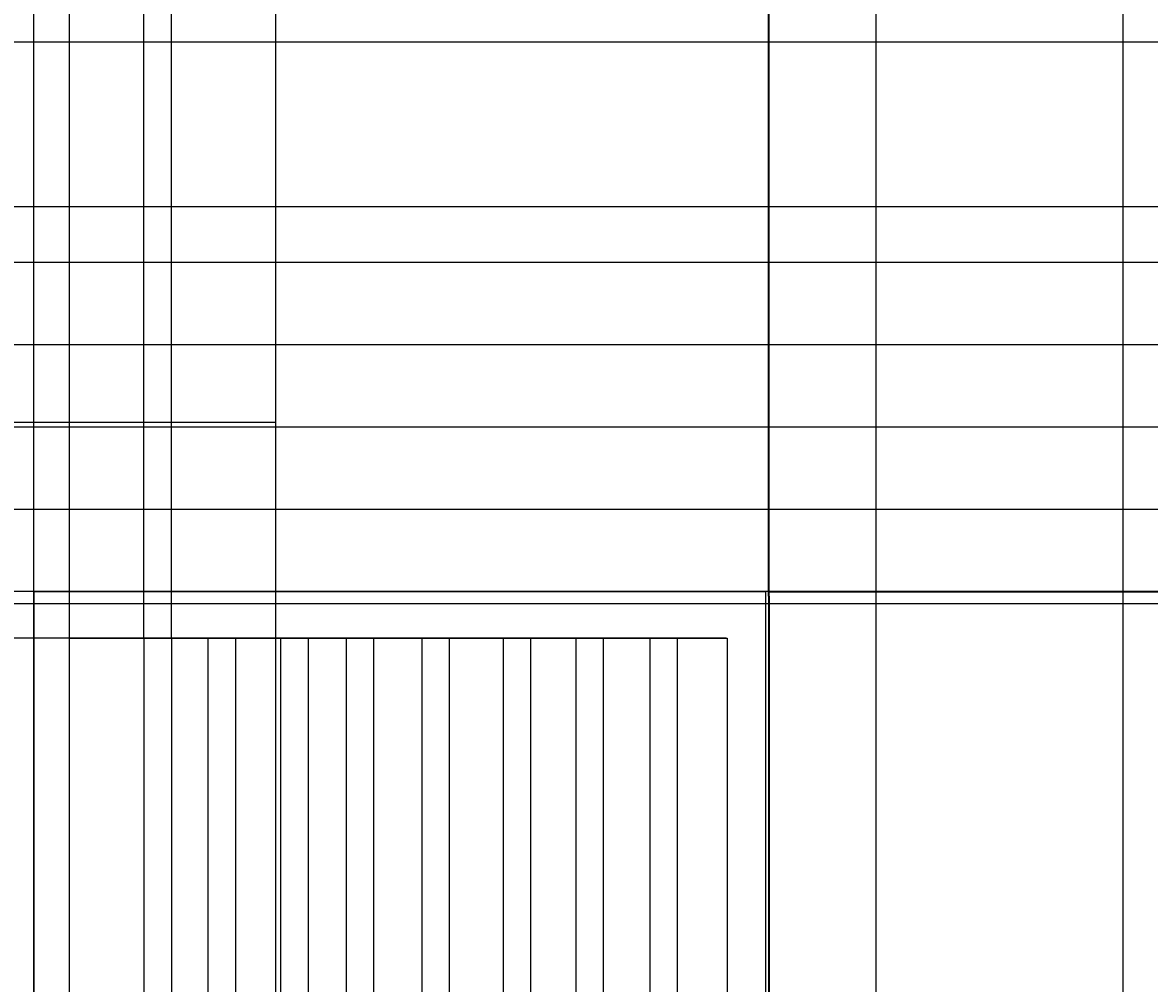
# Model space of a CAD drawing. Units: inches. Extents: x -13 to 809, y 112 to 656.
# Tile 12 of 55: x 257 to 339, y 182 to 252. Entities that reach past the tile are written whole.
import ezdxf

# ---------------------------------------------------------------- set-up
doc = ezdxf.new("R2010")
doc.units = ezdxf.units.IN
doc.header["$MEASUREMENT"] = 0
for name, color, linetype, lineweight in [('A-ANNO-DIMS', 2, 'Continuous', 18), ('A-DOOR', 4, 'Continuous', 25), ('A-ELEV', 7, 'Continuous', 35), ('A-GLAZ', 4, 'Continuous', 25)]:
    doc.layers.add(name, color=color, linetype=linetype, lineweight=lineweight)
doc.styles.get("Standard").update_dxf_attribs({"font": 'arial.ttf'})
doc.dimstyles.get("Standard").update_dxf_attribs({"dimtxt": 0.625, "dimasz": 0.18, "dimexe": 0.18, "dimexo": 0.0625, "dimgap": 0.09, "dimtad": 0, "dimtih": 1, "dimtoh": 1, "dimdec": 4, "dimzin": 0, "dimdsep": 46, "dimlunit": 4, "dimtxsty": 'Standard', "dimcen": 0.09, "dimadec": 0, "dimazin": 0, "dimtfac": 1, "dimtdec": 4, "dimtofl": 0, "dimtmove": 0, "dimatfit": 3, "dimfxl": 1, "dimtolj": 1, "dimtzin": 0, "dimarcsym": 0})

# ---------------------------------------------------------------- blocks, each defined once
blk = doc.blocks.new('*D15')
at = {"layer": 'A-ANNO-DIMS', "color": 0, "lineweight": -2, "transparency": 16777216}
for p, q in [((210.079, 223.038), (210.079, 112.34)), ((258.102, 210.722), (258.102, 112.34)), ((210.259, 112.52), (232.937, 112.52)), ((257.922, 112.52), (235.245, 112.52))]:
    blk.add_line(p, q, dxfattribs=at)
at = {"layer": 'A-ANNO-DIMS', "color": 0, "transparency": 16777216}
for points in [[(210.259, 112.55), (210.259, 112.49), (210.079, 112.52)], [(257.922, 112.55), (257.922, 112.49), (258.102, 112.52)]]:
    blk.add_solid(points, dxfattribs=at)
at = {"layer": 'Defpoints', "color": 0, "transparency": 16777216}
for p in [(210.079, 223.1), (258.102, 210.785), (258.102, 112.52)]:
    blk.add_point(p, dxfattribs=at)
at = {"layer": 'A-ANNO-DIMS', "color": 0, "transparency": 16777216, "insert": (234.091, 112.52), "char_height": 0.625, "attachment_point": 5}
blk.add_mtext('\\A1;48.02', dxfattribs=at)
blk = doc.blocks.new('*D16')
at = {"layer": 'A-ANNO-DIMS', "color": 0, "lineweight": -2, "transparency": 16777216}
for p, q in [((275.715, 223.038), (275.715, 112.34)), ((258.102, 210.722), (258.102, 112.34)), ((258.282, 112.52), (265.554, 112.52)), ((275.535, 112.52), (268.263, 112.52))]:
    blk.add_line(p, q, dxfattribs=at)
at = {"layer": 'A-ANNO-DIMS', "color": 0, "transparency": 16777216}
for points in [[(258.282, 112.55), (258.282, 112.49), (258.102, 112.52)], [(275.535, 112.55), (275.535, 112.49), (275.715, 112.52)]]:
    blk.add_solid(points, dxfattribs=at)
at = {"layer": 'Defpoints', "color": 0, "transparency": 16777216}
for p in [(275.715, 223.1), (258.102, 210.785), (275.715, 112.52)]:
    blk.add_point(p, dxfattribs=at)
at = {"layer": 'A-ANNO-DIMS', "color": 0, "transparency": 16777216, "insert": (266.908, 112.52), "char_height": 0.625, "attachment_point": 5}
blk.add_mtext('\\A1;17.612', dxfattribs=at)
blk = doc.blocks.new('*D17')
at = {"layer": 'A-ANNO-DIMS', "color": 0, "lineweight": -2, "transparency": 16777216}
for p, q in [((275.715, 223.038), (275.715, 112.34)), ((311.463, 210.722), (311.463, 112.34)), ((275.895, 112.52), (292.442, 112.52)), ((311.283, 112.52), (294.735, 112.52))]:
    blk.add_line(p, q, dxfattribs=at)
at = {"layer": 'A-ANNO-DIMS', "color": 0, "transparency": 16777216}
for points in [[(275.895, 112.55), (275.895, 112.49), (275.715, 112.52)], [(311.283, 112.55), (311.283, 112.49), (311.463, 112.52)]]:
    blk.add_solid(points, dxfattribs=at)
at = {"layer": 'Defpoints', "color": 0, "transparency": 16777216}
for p in [(275.715, 223.1), (311.463, 210.785), (311.463, 112.52)]:
    blk.add_point(p, dxfattribs=at)
at = {"layer": 'A-ANNO-DIMS', "color": 0, "transparency": 16777216, "insert": (293.589, 112.52), "char_height": 0.625, "attachment_point": 5}
blk.add_mtext('\\A1;35.75', dxfattribs=at)
blk = doc.blocks.new('*D18')
at = {"layer": 'A-ANNO-DIMS', "color": 0, "lineweight": -2, "transparency": 16777216}
for p, q in [((337.507, 306.457), (337.507, 112.34)), ((311.463, 210.722), (311.463, 112.34)), ((311.643, 112.52), (323.09, 112.52)), ((337.327, 112.52), (325.88, 112.52))]:
    blk.add_line(p, q, dxfattribs=at)
at = {"layer": 'A-ANNO-DIMS', "color": 0, "transparency": 16777216}
for points in [[(311.643, 112.55), (311.643, 112.49), (311.463, 112.52)], [(337.327, 112.55), (337.327, 112.49), (337.507, 112.52)]]:
    blk.add_solid(points, dxfattribs=at)
at = {"layer": 'Defpoints', "color": 0, "transparency": 16777216}
for p in [(337.507, 306.52), (311.463, 210.785), (337.507, 112.52)]:
    blk.add_point(p, dxfattribs=at)
at = {"layer": 'A-ANNO-DIMS', "color": 0, "transparency": 16777216, "insert": (324.485, 112.52), "char_height": 0.625, "attachment_point": 5}
blk.add_mtext('\\A1;26.045', dxfattribs=at)
blk = doc.blocks.new('*D19')
at = {"layer": 'A-ANNO-DIMS', "color": 0, "lineweight": -2, "transparency": 16777216}
for p, q in [((337.507, 306.457), (337.507, 112.34)), ((365.938, 210.722), (365.938, 112.34)), ((337.687, 112.52), (350.573, 112.52)), ((365.758, 112.52), (352.873, 112.52))]:
    blk.add_line(p, q, dxfattribs=at)
at = {"layer": 'A-ANNO-DIMS', "color": 0, "transparency": 16777216}
for points in [[(337.687, 112.55), (337.687, 112.49), (337.507, 112.52)], [(365.758, 112.55), (365.758, 112.49), (365.938, 112.52)]]:
    blk.add_solid(points, dxfattribs=at)
at = {"layer": 'Defpoints', "color": 0, "transparency": 16777216}
for p in [(337.507, 306.52), (365.938, 210.785), (365.938, 112.52)]:
    blk.add_point(p, dxfattribs=at)
at = {"layer": 'A-ANNO-DIMS', "color": 0, "transparency": 16777216, "insert": (351.723, 112.52), "char_height": 0.625, "attachment_point": 5}
blk.add_mtext('\\A1;28.43', dxfattribs=at)
blk = doc.blocks.new('*D45')
at = {"layer": 'A-ANNO-DIMS', "color": 0, "lineweight": -2, "transparency": 16777216}
for p, q in [((275.652, 270.602), (-12.099, 270.602)), ((-11.919, 270.422), (-11.919, 247.259)), ((-11.919, 223.28), (-11.919, 246.443)), ((275.652, 223.1), (-12.099, 223.1))]:
    blk.add_line(p, q, dxfattribs=at)
at = {"layer": 'A-ANNO-DIMS', "color": 0, "transparency": 16777216}
for points in [[(-11.949, 270.422), (-11.889, 270.422), (-11.919, 270.602)], [(-11.949, 223.28), (-11.889, 223.28), (-11.919, 223.1)]]:
    blk.add_solid(points, dxfattribs=at)
at = {"layer": 'Defpoints', "color": 0, "transparency": 16777216}
for p in [(-11.919, 270.602), (275.715, 270.602), (275.715, 223.1)]:
    blk.add_point(p, dxfattribs=at)
at = {"layer": 'A-ANNO-DIMS', "color": 0, "transparency": 16777216, "insert": (-11.919, 246.851), "char_height": 0.625, "attachment_point": 5}
blk.add_mtext('\\A1;47.5', dxfattribs=at)
blk = doc.blocks.new('*D49')
at = {"layer": 'A-ANNO-DIMS', "color": 0, "lineweight": -2, "transparency": 16777216}
for p, q in [((590.946, 250.843), (-12.099, 250.843)), ((-11.919, 250.663), (-11.919, 245.247)), ((-11.919, 239.023), (-11.919, 244.439)), ((590.946, 238.843), (-12.099, 238.843))]:
    blk.add_line(p, q, dxfattribs=at)
at = {"layer": 'A-ANNO-DIMS', "color": 0, "transparency": 16777216}
for points in [[(-11.949, 250.663), (-11.889, 250.663), (-11.919, 250.843)], [(-11.949, 239.023), (-11.889, 239.023), (-11.919, 238.843)]]:
    blk.add_solid(points, dxfattribs=at)
at = {"layer": 'Defpoints', "color": 0, "transparency": 16777216}
for p in [(-11.919, 250.843), (591.008, 250.843), (591.008, 238.843)]:
    blk.add_point(p, dxfattribs=at)
at = {"layer": 'A-ANNO-DIMS', "color": 0, "transparency": 16777216, "insert": (-11.919, 244.843), "char_height": 0.625, "attachment_point": 5}
blk.add_mtext('\\A1;12', dxfattribs=at)
blk = doc.blocks.new('*D50')
at = {"layer": 'A-ANNO-DIMS', "color": 0, "lineweight": -2, "transparency": 16777216}
for p, q in [((590.946, 238.843), (-12.099, 238.843)), ((-11.919, 238.663), (-11.919, 224.768)), ((-11.919, 210.055), (-11.919, 223.95)), ((607.512, 209.875), (-12.099, 209.875))]:
    blk.add_line(p, q, dxfattribs=at)
at = {"layer": 'A-ANNO-DIMS', "color": 0, "transparency": 16777216}
for points in [[(-11.949, 238.663), (-11.889, 238.663), (-11.919, 238.843)], [(-11.949, 210.055), (-11.889, 210.055), (-11.919, 209.875)]]:
    blk.add_solid(points, dxfattribs=at)
at = {"layer": 'Defpoints', "color": 0, "transparency": 16777216}
for p in [(591.008, 238.843), (-11.919, 209.875), (607.574, 209.875)]:
    blk.add_point(p, dxfattribs=at)
at = {"layer": 'A-ANNO-DIMS', "color": 0, "transparency": 16777216, "insert": (-11.919, 224.359), "char_height": 0.625, "attachment_point": 5}
blk.add_mtext('\\A1;28.97', dxfattribs=at)
blk = doc.blocks.new('*D80')
at = {"layer": 'A-ANNO-DIMS', "color": 0, "lineweight": -2, "transparency": 16777216}
for p, q in [((368.834, 216.774), (-12.099, 216.774)), ((-11.919, 216.594), (-11.919, 214.183)), ((-11.919, 210.954), (-11.919, 213.365)), ((368.834, 210.774), (-12.099, 210.774))]:
    blk.add_line(p, q, dxfattribs=at)
at = {"layer": 'A-ANNO-DIMS', "color": 0, "transparency": 16777216}
for points in [[(-11.949, 216.594), (-11.889, 216.594), (-11.919, 216.774)], [(-11.949, 210.954), (-11.889, 210.954), (-11.919, 210.774)]]:
    blk.add_solid(points, dxfattribs=at)
at = {"layer": 'Defpoints', "color": 0, "transparency": 16777216}
for p in [(-11.919, 216.774), (368.897, 216.774), (368.897, 210.774)]:
    blk.add_point(p, dxfattribs=at)
at = {"layer": 'A-ANNO-DIMS', "color": 0, "transparency": 16777216, "insert": (-11.919, 213.774), "char_height": 0.625, "attachment_point": 5}
blk.add_mtext('\\A1;6', dxfattribs=at)
blk = doc.blocks.new('*D81')
at = {"layer": 'A-ANNO-DIMS', "color": 0, "lineweight": -2, "transparency": 16777216}
for p, q in [((378.834, 222.774), (-12.099, 222.774)), ((-11.919, 222.594), (-11.919, 220.183)), ((-11.919, 216.954), (-11.919, 219.365)), ((378.834, 216.774), (-12.099, 216.774))]:
    blk.add_line(p, q, dxfattribs=at)
at = {"layer": 'A-ANNO-DIMS', "color": 0, "transparency": 16777216}
for points in [[(-11.949, 222.594), (-11.889, 222.594), (-11.919, 222.774)], [(-11.949, 216.954), (-11.889, 216.954), (-11.919, 216.774)]]:
    blk.add_solid(points, dxfattribs=at)
at = {"layer": 'Defpoints', "color": 0, "transparency": 16777216}
for p in [(-11.919, 222.774), (378.897, 222.774), (378.897, 216.774)]:
    blk.add_point(p, dxfattribs=at)
at = {"layer": 'A-ANNO-DIMS', "color": 0, "transparency": 16777216, "insert": (-11.919, 219.774), "char_height": 0.625, "attachment_point": 5}
blk.add_mtext('\\A1;6', dxfattribs=at)
blk = doc.blocks.new('*D82')
at = {"layer": 'A-ANNO-DIMS', "color": 0, "lineweight": -2, "transparency": 16777216}
for p, q in [((388.834, 228.774), (-12.099, 228.774)), ((-11.919, 228.594), (-11.919, 226.183)), ((-11.919, 222.954), (-11.919, 225.365)), ((388.834, 222.774), (-12.099, 222.774))]:
    blk.add_line(p, q, dxfattribs=at)
at = {"layer": 'A-ANNO-DIMS', "color": 0, "transparency": 16777216}
for points in [[(-11.949, 228.594), (-11.889, 228.594), (-11.919, 228.774)], [(-11.949, 222.954), (-11.889, 222.954), (-11.919, 222.774)]]:
    blk.add_solid(points, dxfattribs=at)
at = {"layer": 'Defpoints', "color": 0, "transparency": 16777216}
for p in [(-11.919, 228.774), (388.897, 228.774), (388.897, 222.774)]:
    blk.add_point(p, dxfattribs=at)
at = {"layer": 'A-ANNO-DIMS', "color": 0, "transparency": 16777216, "insert": (-11.919, 225.774), "char_height": 0.625, "attachment_point": 5}
blk.add_mtext('\\A1;6', dxfattribs=at)
blk = doc.blocks.new('*D83')
at = {"layer": 'A-ANNO-DIMS', "color": 0, "lineweight": -2, "transparency": 16777216}
for p, q in [((398.834, 234.774), (-12.099, 234.774)), ((-11.919, 234.594), (-11.919, 232.183)), ((-11.919, 228.954), (-11.919, 231.365)), ((398.834, 228.774), (-12.099, 228.774))]:
    blk.add_line(p, q, dxfattribs=at)
at = {"layer": 'A-ANNO-DIMS', "color": 0, "transparency": 16777216}
for points in [[(-11.949, 234.594), (-11.889, 234.594), (-11.919, 234.774)], [(-11.949, 228.954), (-11.889, 228.954), (-11.919, 228.774)]]:
    blk.add_solid(points, dxfattribs=at)
at = {"layer": 'Defpoints', "color": 0, "transparency": 16777216}
for p in [(-11.919, 234.774), (398.897, 234.774), (398.897, 228.774)]:
    blk.add_point(p, dxfattribs=at)
at = {"layer": 'A-ANNO-DIMS', "color": 0, "transparency": 16777216, "insert": (-11.919, 231.774), "char_height": 0.625, "attachment_point": 5}
blk.add_mtext('\\A1;6', dxfattribs=at)
blk = doc.blocks.new('*D84')
at = {"layer": 'A-ANNO-DIMS', "color": 0, "lineweight": -2, "transparency": 16777216}
for p, q in [((408.834, 238.843), (-12.099, 238.843)), ((-11.919, 238.663), (-11.919, 237.217)), ((-11.919, 234.954), (-11.919, 236.399)), ((408.834, 234.774), (-12.099, 234.774))]:
    blk.add_line(p, q, dxfattribs=at)
at = {"layer": 'A-ANNO-DIMS', "color": 0, "transparency": 16777216}
for points in [[(-11.949, 238.663), (-11.889, 238.663), (-11.919, 238.843)], [(-11.949, 234.954), (-11.889, 234.954), (-11.919, 234.774)]]:
    blk.add_solid(points, dxfattribs=at)
at = {"layer": 'Defpoints', "color": 0, "transparency": 16777216}
for p in [(-11.919, 238.843), (408.897, 238.843), (408.897, 234.774)]:
    blk.add_point(p, dxfattribs=at)
at = {"layer": 'A-ANNO-DIMS', "color": 0, "transparency": 16777216, "insert": (-11.919, 236.808), "char_height": 0.625, "attachment_point": 5}
blk.add_mtext('\\A1;4.069', dxfattribs=at)
blk = doc.blocks.new('*D108')
at = {"layer": 'A-ANNO-DIMS', "color": 0, "lineweight": -2, "transparency": 16777216}
for p, q in [((319.507, 324.457), (319.507, 112.34)), ((337.507, 306.457), (337.507, 112.34)), ((319.687, 112.52), (327.393, 112.52)), ((337.327, 112.52), (329.621, 112.52))]:
    blk.add_line(p, q, dxfattribs=at)
at = {"layer": 'A-ANNO-DIMS', "color": 0, "transparency": 16777216}
for points in [[(319.687, 112.55), (319.687, 112.49), (319.507, 112.52)], [(337.327, 112.55), (337.327, 112.49), (337.507, 112.52)]]:
    blk.add_solid(points, dxfattribs=at)
at = {"layer": 'Defpoints', "color": 0, "transparency": 16777216}
for p in [(319.507, 324.52), (337.507, 306.52), (337.507, 112.52)]:
    blk.add_point(p, dxfattribs=at)
at = {"layer": 'A-ANNO-DIMS', "color": 0, "transparency": 16777216, "insert": (328.507, 112.52), "char_height": 0.625, "attachment_point": 5}
blk.add_mtext('\\A1;18.00', dxfattribs=at)
blk = doc.blocks.new('*D112')
at = {"layer": 'A-ANNO-DIMS', "color": 0, "lineweight": -2, "transparency": 16777216}
for p, q in [((210.079, 361.229), (210.079, 112.34)), ((275.715, 361.229), (275.715, 112.34)), ((210.259, 112.52), (241.752, 112.52)), ((275.535, 112.52), (244.042, 112.52))]:
    blk.add_line(p, q, dxfattribs=at)
at = {"layer": 'A-ANNO-DIMS', "color": 0, "transparency": 16777216}
for points in [[(210.259, 112.55), (210.259, 112.49), (210.079, 112.52)], [(275.535, 112.55), (275.535, 112.49), (275.715, 112.52)]]:
    blk.add_solid(points, dxfattribs=at)
at = {"layer": 'Defpoints', "color": 0, "transparency": 16777216}
for p in [(210.079, 361.292), (275.715, 361.292), (275.715, 112.52)]:
    blk.add_point(p, dxfattribs=at)
at = {"layer": 'A-ANNO-DIMS', "color": 0, "transparency": 16777216, "insert": (242.897, 112.52), "char_height": 0.625, "attachment_point": 5}
blk.add_mtext('\\A1;65.64', dxfattribs=at)
blk = doc.blocks.new('*D113')
at = {"layer": 'A-ANNO-DIMS', "color": 0, "lineweight": -2, "transparency": 16777216}
for p, q in [((275.715, 361.229), (275.715, 112.34)), ((319.507, 324.457), (319.507, 112.34)), ((275.895, 112.52), (296.453, 112.52)), ((319.327, 112.52), (298.769, 112.52))]:
    blk.add_line(p, q, dxfattribs=at)
at = {"layer": 'A-ANNO-DIMS', "color": 0, "transparency": 16777216}
for points in [[(275.895, 112.55), (275.895, 112.49), (275.715, 112.52)], [(319.327, 112.55), (319.327, 112.49), (319.507, 112.52)]]:
    blk.add_solid(points, dxfattribs=at)
at = {"layer": 'Defpoints', "color": 0, "transparency": 16777216}
for p in [(275.715, 361.292), (319.507, 324.52), (319.507, 112.52)]:
    blk.add_point(p, dxfattribs=at)
at = {"layer": 'A-ANNO-DIMS', "color": 0, "transparency": 16777216, "insert": (297.611, 112.52), "char_height": 0.625, "attachment_point": 5}
blk.add_mtext('\\A1;43.79', dxfattribs=at)
blk = doc.blocks.new('*D115')
at = {"layer": 'A-ANNO-DIMS', "color": 0, "lineweight": -2, "transparency": 16777216}
for p, q in [((311.4, 210.785), (-12.099, 210.785)), ((-11.919, 210.605), (-11.919, 181.062)), ((-11.919, 150.7), (-11.919, 180.243)), ((311.637, 150.52), (-12.099, 150.52))]:
    blk.add_line(p, q, dxfattribs=at)
at = {"layer": 'A-ANNO-DIMS', "color": 0, "transparency": 16777216}
for points in [[(-11.949, 210.605), (-11.889, 210.605), (-11.919, 210.785)], [(-11.949, 150.7), (-11.889, 150.7), (-11.919, 150.52)]]:
    blk.add_solid(points, dxfattribs=at)
at = {"layer": 'Defpoints', "color": 0, "transparency": 16777216}
for p in [(-11.919, 210.785), (311.463, 210.785), (311.699, 150.52)]:
    blk.add_point(p, dxfattribs=at)
at = {"layer": 'A-ANNO-DIMS', "color": 0, "transparency": 16777216, "insert": (-11.919, 180.652), "char_height": 0.625, "attachment_point": 5}
blk.add_mtext('\\A1;60.27', dxfattribs=at)
blk = doc.blocks.new('*D116')
at = {"layer": 'A-ANNO-DIMS', "color": 0, "lineweight": -2, "transparency": 16777216}
for p, q in [((258.102, 210.847), (258.102, 655.963)), ((260.705, 207.435), (260.705, 655.963)), ((258.282, 655.783), (258.497, 655.783)), ((260.525, 655.783), (260.309, 655.783))]:
    blk.add_line(p, q, dxfattribs=at)
at = {"layer": 'A-ANNO-DIMS', "color": 0, "transparency": 16777216}
for points in [[(258.282, 655.813), (258.282, 655.753), (258.102, 655.783)], [(260.525, 655.813), (260.525, 655.753), (260.705, 655.783)]]:
    blk.add_solid(points, dxfattribs=at)
at = {"layer": 'Defpoints', "color": 0, "transparency": 16777216}
for p in [(260.705, 655.783), (258.102, 210.785), (260.705, 207.372)]:
    blk.add_point(p, dxfattribs=at)
at = {"layer": 'A-ANNO-DIMS', "color": 0, "transparency": 16777216, "insert": (259.403, 655.783), "char_height": 0.625, "attachment_point": 5}
blk.add_mtext('\\A1;2.60', dxfattribs=at)
blk = doc.blocks.new('*D118')
at = {"layer": 'A-ANNO-DIMS', "color": 0, "lineweight": -2, "transparency": 16777216}
for p, q in [((311.4, 210.785), (-12.099, 210.785)), ((-11.919, 210.605), (-11.919, 209.488)), ((-11.919, 207.552), (-11.919, 208.669)), ((308.586, 207.372), (-12.099, 207.372))]:
    blk.add_line(p, q, dxfattribs=at)
at = {"layer": 'A-ANNO-DIMS', "color": 0, "transparency": 16777216}
for points in [[(-11.949, 210.605), (-11.889, 210.605), (-11.919, 210.785)], [(-11.949, 207.552), (-11.889, 207.552), (-11.919, 207.372)]]:
    blk.add_solid(points, dxfattribs=at)
at = {"layer": 'Defpoints', "color": 0, "transparency": 16777216}
for p in [(-11.919, 210.785), (311.463, 210.785), (308.649, 207.372)]:
    blk.add_point(p, dxfattribs=at)
at = {"layer": 'A-ANNO-DIMS', "color": 0, "transparency": 16777216, "insert": (-11.919, 209.079), "char_height": 0.625, "attachment_point": 5}
blk.add_mtext('\\A1;3.41', dxfattribs=at)
blk = doc.blocks.new('*D119')
at = {"layer": 'A-ANNO-DIMS', "color": 0, "lineweight": -2, "transparency": 16777216}
for p, q in [((266.1286, 207.43492), (266.1286, 655.962835)), ((268.1286, 207.43492), (268.1286, 655.962835)), ((265.9486, 655.782835), (265.7686, 655.782835)), ((268.3086, 655.782835), (268.4886, 655.782835))]:
    blk.add_line(p, q, dxfattribs=at)
at = {"layer": 'A-ANNO-DIMS', "color": 0, "transparency": 16777216}
for points in [[(265.9486, 655.812835), (265.9486, 655.752835), (266.1286, 655.782835)], [(268.3086, 655.812835), (268.3086, 655.752835), (268.1286, 655.782835)]]:
    blk.add_solid(points, dxfattribs=at)
at = {"layer": 'Defpoints', "color": 0, "transparency": 16777216}
for p in [(268.1286, 655.782835), (266.1286, 207.37242), (268.1286, 207.37242)]:
    blk.add_point(p, dxfattribs=at)
at = {"layer": 'A-ANNO-DIMS', "color": 0, "transparency": 16777216, "insert": (267.1286, 655.782835), "char_height": 0.625, "attachment_point": 5}
blk.add_mtext('\\A1;2.00', dxfattribs=at)

msp = doc.modelspace()

# ---------------------------------------------------------------- linework, layer by layer
at = {"layer": 'A-DOOR'}
for p, q in [((266.1286, 207.3724), (266.1286, 154.2723)), ((268.1286, 207.3724), (268.1286, 154.2723)), ((270.7975, 207.3724), (270.7975, 154.2723)), ((272.7975, 207.3724), (272.7975, 154.2723)), ((276.0927, 207.3724), (276.0927, 154.2723)), ((278.0927, 207.3724), (278.0927, 154.2723)), ((280.8755, 207.3724), (280.8755, 154.2723)), ((282.8755, 207.3724), (282.8755, 154.2723)), ((286.3985, 207.3724), (286.3985, 154.2723)), ((288.3985, 207.3724), (288.3985, 154.2723)), ((292.32, 207.3724), (292.32, 154.2723)), ((294.32, 207.3724), (294.32, 154.2723)), ((297.6152, 207.3724), (297.6152, 154.2723)), ((299.6152, 207.3724), (299.6152, 154.2723)), ((303.0243, 207.3724), (303.0243, 154.2723)), ((305.0243, 207.3724), (305.0243, 154.2723))]:
    msp.add_line(p, q, dxfattribs=at)
for points in [[(258.1022, 210.7849), (311.4627, 210.7849), (311.4627, 150.7849), (258.1022, 150.7849)], [(260.7048, 207.3724), (308.6488, 207.3724), (308.6488, 154.2723), (260.7048, 154.2723)]]:
    msp.add_lwpolyline(points, close=True, dxfattribs=at)
at = {"layer": 'A-ELEV'}
for p, q in [((311.6991, 210.4452), (311.6991, 306.5199)), ((311.6991, 210.7849), (363.3158, 210.7849)), ((311.6991, 210.4452), (311.6991, 150.5199))]:
    msp.add_line(p, q, dxfattribs=at)
at = {"layer": 'A-GLAZ'}
msp.add_lwpolyline([(210.0791, 270.6024), (275.7145, 270.6024), (275.7145, 223.1), (210.0791, 223.1)], close=True, dxfattribs=at)

# ---------------------------------------------------------------- dimensions: what is measured, and where the dimension line sits
at = {"layer": 'A-ANNO-DIMS'}
for base, p1, p2, override, picture, middle in [((260.7048, 655.7828), (258.1022, 210.7849), (260.7048, 207.3724), {"dimdec": 2, "dimlfac": 1, "dimrnd": 0, "dimzin": 0, "dimdsep": 46, "dimlunit": 2}, '*D116', (259.4035, 655.7828)), ((268.1286, 655.7828), (266.1286, 207.3724), (268.1286, 207.3724), {"dimdec": 2, "dimlfac": 1, "dimrnd": 0, "dimzin": 0, "dimdsep": 46, "dimlunit": 2}, '*D119', (267.1286, 655.7828)), ((275.7145, 112.5199), (210.0791, 361.2915), (275.7145, 361.2915), {"dimdec": 2, "dimlfac": 1, "dimrnd": 0, "dimzin": 0, "dimdsep": 46, "dimlunit": 2}, '*D112', (242.8968, 112.5199)), ((319.5074, 112.5199), (275.7145, 361.2915), (319.5074, 324.5199), {"dimdec": 2, "dimlfac": 1, "dimrnd": 0, "dimzin": 0, "dimdsep": 46, "dimlunit": 2}, '*D113', (297.611, 112.5199)), ((337.5074, 112.5199), (319.5074, 324.5199), (337.5074, 306.5199), {"dimdec": 2, "dimlfac": 1, "dimrnd": 0, "dimzin": 0, "dimdsep": 46, "dimlunit": 2}, '*D108', (328.5074, 112.5199)), ((337.5074, 112.5199), (311.4627, 210.7849), (337.5074, 306.5199), {"dimdec": 3, "dimlfac": 1, "dimrnd": 0, "dimzin": 0, "dimdsep": 46, "dimlunit": 2}, '*D18', (324.4851, 112.5199)), ((365.9383, 112.5199), (337.5074, 306.5199), (365.9383, 210.7849), {"dimdec": 2, "dimlfac": 1, "dimrnd": 0, "dimzin": 0, "dimdsep": 46, "dimlunit": 2}, '*D19', (351.7228, 112.5199)), ((258.1022, 112.5199), (210.0791, 223.1), (258.1022, 210.7849), {"dimdec": 2, "dimlfac": 1, "dimrnd": 0, "dimzin": 0, "dimdsep": 46, "dimlunit": 2}, '*D15', (234.0906, 112.5199)), ((275.7145, 112.5199), (258.1022, 210.7849), (275.7145, 223.1), {"dimdec": 3, "dimlfac": 1, "dimrnd": 0, "dimzin": 0, "dimdsep": 46, "dimlunit": 2}, '*D16', (266.9083, 112.5199)), ((311.4627, 112.5199), (275.7145, 223.1), (311.4627, 210.7849), {"dimdec": 2, "dimlfac": 1, "dimrnd": 0, "dimzin": 0, "dimdsep": 46, "dimlunit": 2}, '*D17', (293.5886, 112.5199))]:
    dim = msp.add_linear_dim(base=base, p1=p1, p2=p2, dimstyle='Standard', override=override, dxfattribs=at)
    dim.commit()
    dim.dimension.update_dxf_attribs({"geometry": picture, "text_midpoint": middle})
for base, p1, p2, override, picture, middle in [((-11.9191, 270.6024), (275.7145, 223.1), (275.7145, 270.6024), {"dimdec": 1, "dimlfac": 1, "dimrnd": 0, "dimzin": 0, "dimdsep": 46, "dimlunit": 2}, '*D45', (-11.9191, 246.8512)), ((-11.9191, 250.8429), (591.008, 238.8429), (591.008, 250.8429), {"dimdec": 0, "dimlfac": 1, "dimrnd": 0, "dimzin": 0, "dimdsep": 46, "dimlunit": 2}, '*D49', (-11.9191, 244.8429)), ((-11.9191, 209.8753), (591.008, 238.8429), (607.5741, 209.8753), {"dimdec": 2, "dimlfac": 1, "dimrnd": 0, "dimzin": 0, "dimdsep": 46, "dimlunit": 2}, '*D50', (-11.9191, 224.3591)), ((-11.9191, 238.8429), (408.8966, 234.7738), (408.8966, 238.8429), {"dimdec": 3, "dimlfac": 1, "dimrnd": 0, "dimzin": 0, "dimdsep": 46, "dimlunit": 2}, '*D84', (-11.9191, 236.8083)), ((-11.9191, 234.7738), (398.8966, 228.7738), (398.8966, 234.7738), {"dimdec": 0, "dimlfac": 1, "dimrnd": 0, "dimzin": 0, "dimdsep": 46, "dimlunit": 2}, '*D83', (-11.9191, 231.7738)), ((-11.9191, 228.7738), (388.8966, 222.7738), (388.8966, 228.7738), {"dimdec": 0, "dimlfac": 1, "dimrnd": 0, "dimzin": 0, "dimdsep": 46, "dimlunit": 2}, '*D82', (-11.9191, 225.7738)), ((-11.9191, 222.7738), (378.8966, 216.7738), (378.8966, 222.7738), {"dimdec": 0, "dimlfac": 1, "dimrnd": 0, "dimzin": 0, "dimdsep": 46, "dimlunit": 2}, '*D81', (-11.9191, 219.7738)), ((-11.9191, 216.7738), (368.8966, 210.7738), (368.8966, 216.7738), {"dimdec": 0, "dimlfac": 1, "dimrnd": 0, "dimzin": 0, "dimdsep": 46, "dimlunit": 2}, '*D80', (-11.9191, 213.7738)), ((-11.91915, 210.78493), (311.6991, 150.51989), (311.46269, 210.78493), {"dimdec": 2, "dimlfac": 1, "dimrnd": 0, "dimzin": 0, "dimdsep": 46, "dimlunit": 2}, '*D115', (-11.91915, 180.65241)), ((-11.9191, 210.7849), (308.6488, 207.3724), (311.4627, 210.7849), {"dimdec": 2, "dimlfac": 1, "dimrnd": 0, "dimzin": 0, "dimdsep": 46, "dimlunit": 2}, '*D118', (-11.9191, 209.0787))]:
    dim = msp.add_linear_dim(base=base, p1=p1, p2=p2, angle=90, dimstyle='Standard', override=override, dxfattribs=at)
    dim.commit()
    dim.dimension.update_dxf_attribs({"geometry": picture, "text_midpoint": middle})

doc.saveas('drawing.dxf')
